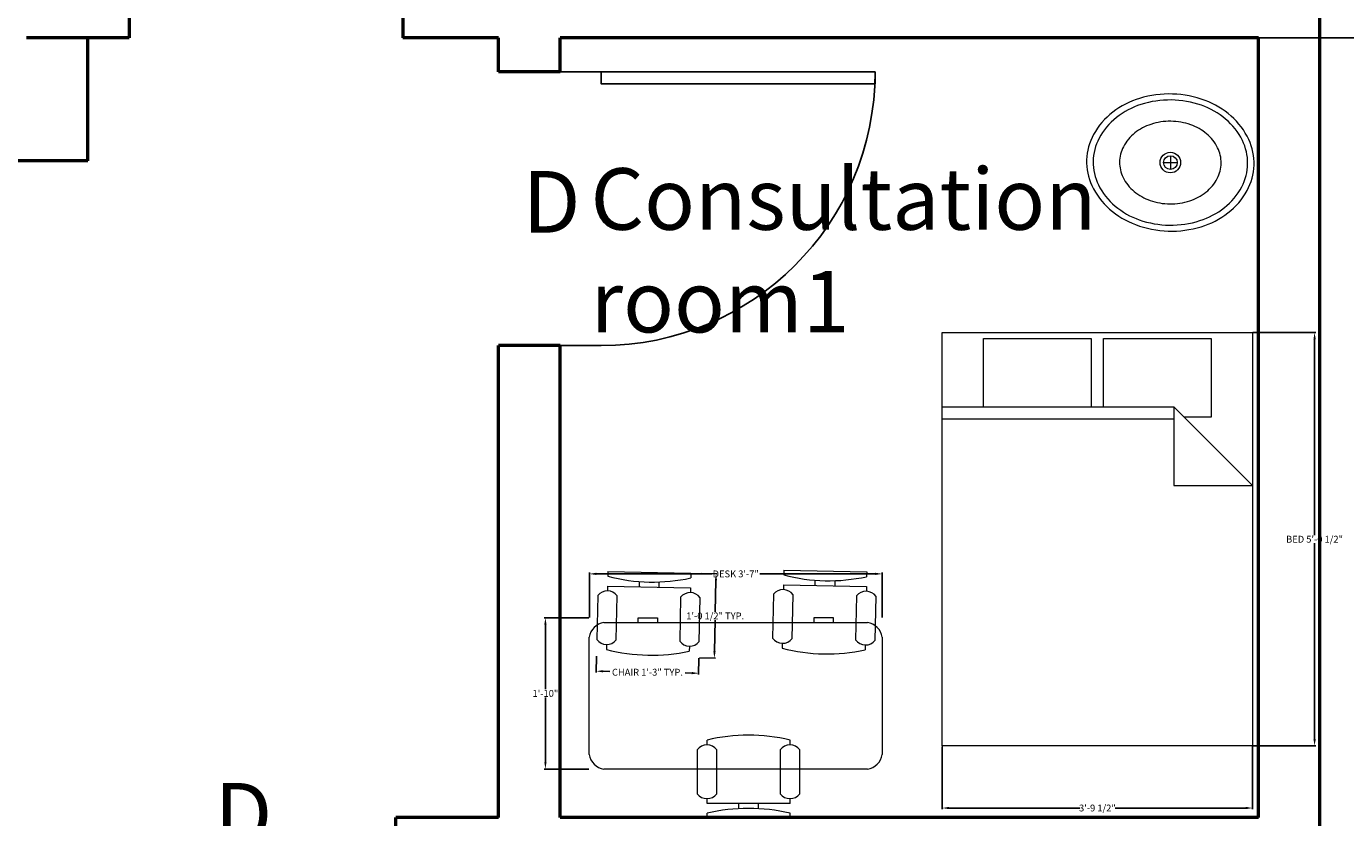
# Model space of a CAD drawing. Units: inches. Extents: x -364 to 705, y -52 to 1250.
# Tile 17 of 34: x 359 to 551, y 417 to 533. Entities that reach past the tile are written whole.
import ezdxf

# ---------------------------------------------------------------- set-up
doc = ezdxf.new("R2010")
doc.units = ezdxf.units.IN
doc.header["$MEASUREMENT"] = 0
for name, color, linetype, lineweight in [('A-ANNO-DIMS', 4, 'Continuous', 18), ('A-ANNO-IDEN', 1, 'Continuous', 18), ('A-AREA-IDEN', 3, 'Continuous', 18), ('A-DOOR', 1, 'Continuous', 25), ('A-FLOR-FIXT', 9, 'Continuous', 18), ('A-FURN', 8, 'Continuous', 18), ('A-WALL', 41, 'Continuous', 50)]:
    doc.layers.add(name, color=color, linetype=linetype, lineweight=lineweight)
doc.styles.get("Standard").update_dxf_attribs({"font": 'arial.ttf'})
doc.dimstyles.get("Standard").update_dxf_attribs({"dimtxt": 1, "dimasz": 1, "dimexe": 0.18, "dimexo": 0.0625, "dimgap": 0.09, "dimtad": 0, "dimtih": 1, "dimtoh": 1, "dimdec": 0, "dimzin": 0, "dimdsep": 46, "dimlunit": 3, "dimtxsty": 'Standard', "dimcen": 0.09, "dimadec": 0, "dimazin": 0, "dimtfac": 1, "dimtdec": 0, "dimtofl": 0, "dimtmove": 0, "dimatfit": 3, "dimfxl": 1, "dimtolj": 1, "dimtzin": 0, "dimarcsym": 0})

# ---------------------------------------------------------------- blocks, each defined once
blk = doc.blocks.new('*U10')
for p, q in [((-40, 0), (-40, 6)), ((0, 0), (0, 6))]:
    blk.add_line(p, q)
blk.add_lwpolyline([(0, 0), (0, -40), (-1.75, -40), (-1.75, 0)], close=True)
blk.add_arc((0, 0), 40, 180, 270)
blk = doc.blocks.new('Chair - Desk')
for p, q in [((-8.5, 0), (-8.5, -1)), ((-8.5, 0), (8.5, 0)), ((8.5, 0), (8.5, -1)), ((-2, -3), (-2, -1.9355)), ((2, -1.9576), (2, -3)), ((-10.5, -5), (-10.5, -14)), ((-8.5, -3), (-8.5, -4)), ((-8.5, -3), (8.5, -3)), ((-6.5, -14), (-6.5, -5)), ((6.5, -5), (6.5, -14)), ((8.5, -3), (8.5, -4)), ((10.5, -14), (10.5, -5)), ((-8.5, -15), (-8.5, -16)), ((8.5, -15), (8.5, -16))]:
    blk.add_line(p, q)
for centre, radius, start, end in [((0, 34.625), 36.625, 256.5803, 283.4197), ((-8.5, -6.5), 2.5, 36.8699, 143.1301), ((8.5, -6.5), 2.5, 36.8699, 143.1301), ((-8.5, -12.5), 2.5, 216.8699, 323.1301), ((0, 19.625), 36.625, 256.5803, 283.4197), ((8.5, -12.5), 2.5, 216.8699, 323.1301)]:
    blk.add_arc(centre, radius, start, end)
blk = doc.blocks.new('Desk - 30 x 60 in.')
for p, q in [((-26.999995, 0), (26.999995, 0)), ((-29.999995, -27), (-29.999995, -3)), ((29.999995, -3), (29.999995, -27)), ((26.999995, -30), (-26.999995, -30)), ((-20.000005, -30), (-20.000005, -31)), ((-20.000005, -31), (-16.000005, -31)), ((-16.000005, -31), (-16.000005, -30)), ((15.999995, -31), (15.999995, -30)), ((19.999995, -31), (15.999995, -31)), ((19.999995, -30), (19.999995, -31))]:
    blk.add_line(p, q)
for centre, start, end in [((-26.499995, -3.5), 98.1301, 171.8699), ((26.499995, -3.5), 8.130102, 81.8699), ((-26.499995, -26.5), 188.1301, 261.8699), ((26.499995, -26.5), 278.1301, 351.8699)]:
    blk.add_arc(centre, 3.535534, start, end)
blk = doc.blocks.new('Bed - Queen')
for p, q in [((0, -80.00003), (0, 0)), ((0, 0), (59.99999, 0)), ((59.99999, 0), (59.99999, -80.00003)), ((7.99999, -1.2), (28.79998, -1.2)), ((7.99999, -14.4), (7.99999, -1.2)), ((28.79998, -1.2), (28.79998, -14.4)), ((31.19999, -1.2), (51.99999, -1.2)), ((31.19999, -14.4), (31.19999, -1.2)), ((51.99999, -1.2), (51.99999, -16.4)), ((0, -14.4), (44.8, -14.4)), ((59.99999, -29.6), (44.8, -14.4)), ((44.8, -14.4), (44.8, -29.6)), ((44.8, -16.8), (0, -16.8)), ((51.99999, -16.4), (46.79936, -16.4)), ((44.8, -29.6), (59.99999, -29.6)), ((59.99999, -80.00003), (0, -80.00003))]:
    blk.add_line(p, q)
blk = doc.blocks.new('Sink - Oval top')
for p, q in [((-1, 0), (1, 0)), ((0, 1), (0, -1))]:
    blk.add_line(p, q)
for points in [[(-12.23, 0.39, 0.117634), (-11.46, -3.36, 0.104469), (-8.88, -6.8, 0.090016), (-5.08, -9.07, 0.08192), (-0.32, -10.02, 0.08192), (4.49, -9.38, 0.090016), (8.42, -7.36, 0.104469), (11.22, -4.09, 0.117634), (12.23, -0.39, 0.117634), (11.46, 3.36, 0.104469), (8.88, 6.8, 0.090016), (5.08, 9.07, 0.08192), (0.32, 10.02, 0.08192), (-4.49, 9.38, 0.090016), (-8.42, 7.36, 0.104469), (-11.22, 4.09, 0.117634)], [(-11.29, 0.16, 0.118622), (-10.52, -3.25, 0.104678), (-8.07, -6.36, 0.089562), (-4.54, -8.37, 0.081185), (-0.13, -9.15, 0.081185), (4.3, -8.49, 0.089562), (7.89, -6.58, 0.104678), (10.42, -3.55, 0.118622), (11.29, -0.16, 0.118622), (10.52, 3.25, 0.104678), (8.07, 6.36, 0.089562), (4.54, 8.37, 0.081185), (0.13, 9.15, 0.081185), (-4.3, 8.49, 0.089562), (-7.89, 6.58, 0.104678), (-10.42, 3.55, 0.118622)], [(-7.42, 0.08, 0.118283), (-6.91, -2.17, 0.104607), (-5.29, -4.21, 0.089718), (-2.97, -5.53, 0.081436), (-0.07, -6.04, 0.081436), (2.84, -5.59, 0.089718), (5.2, -4.33, 0.104607), (6.86, -2.32, 0.118283), (7.42, -0.08, 0.118283), (6.91, 2.17, 0.104607), (5.29, 4.21, 0.089718), (2.97, 5.53, 0.081436), (0.07, 6.04, 0.081436), (-2.84, 5.59, 0.089718), (-5.2, 4.33, 0.104607), (-6.86, 2.32, 0.118283)]]:
    blk.add_lwpolyline(points, format="xyb", close=True)
for radius in [1.5, 1]:
    blk.add_circle((0, 0), radius)
blk = doc.blocks.new('*D38')
at = {"layer": 'A-ANNO-DIMS', "color": 0, "lineweight": -2, "transparency": 16777216}
for p, q in [((441.88, 440.71), (441.83, 438.34)), ((456.85, 440.4), (456.8, 438.04)), ((442.83, 438.5), (443.82, 438.48)), ((455.8, 438.24), (454.82, 438.26))]:
    blk.add_line(p, q, dxfattribs=at)
at = {"layer": 'A-ANNO-DIMS', "color": 0, "transparency": 16777216}
for points in [[(442.83, 438.67), (442.83, 438.34), (441.83, 438.52)], [(455.81, 438.41), (455.8, 438.07), (456.8, 438.22)]]:
    blk.add_solid(points, dxfattribs=at)
at = {"layer": 'Defpoints', "color": 0, "transparency": 16777216}
for p in [(441.88, 440.77), (456.85, 440.47), (456.8, 438.22)]:
    blk.add_point(p, dxfattribs=at)
at = {"layer": 'A-ANNO-DIMS', "color": 0, "transparency": 16777216, "insert": (449.32, 438.37), "char_height": 1, "attachment_point": 5}
blk.add_mtext('\\A1;CHAIR 1\'-3" TYP.', dxfattribs=at)
blk = doc.blocks.new('*D39')
at = {"layer": 'A-ANNO-DIMS', "color": 0, "lineweight": -2, "transparency": 16777216}
for p, q in [((457.16, 452.82), (459.53, 452.77)), ((459.33, 451.78), (459.23, 447.21)), ((459.12, 441.42), (459.21, 445.99)), ((456.91, 440.46), (459.28, 440.42))]:
    blk.add_line(p, q, dxfattribs=at)
at = {"layer": 'A-ANNO-DIMS', "color": 0, "transparency": 16777216}
for points in [[(459.16, 451.78), (459.49, 451.78), (459.35, 452.78)], [(458.95, 441.42), (459.28, 441.42), (459.1, 440.42)]]:
    blk.add_solid(points, dxfattribs=at)
at = {"layer": 'Defpoints', "color": 0, "transparency": 16777216}
for p in [(457.1, 452.82), (459.35, 452.78), (456.85, 440.47)]:
    blk.add_point(p, dxfattribs=at)
at = {"layer": 'A-ANNO-DIMS', "color": 0, "transparency": 16777216, "insert": (459.22, 446.6), "char_height": 1, "attachment_point": 5}
blk.add_mtext('\\A1;1\'-0 1/2" TYP.', dxfattribs=at)
blk = doc.blocks.new('*D48')
at = {"layer": 'A-ANNO-DIMS', "color": 0, "lineweight": -2, "transparency": 16777216}
for p, q in [((440.83, 446.39), (440.83, 452.92)), ((441.83, 452.74), (458.73, 452.74)), ((482.62, 452.74), (465.72, 452.74)), ((483.62, 446.39), (483.62, 452.92))]:
    blk.add_line(p, q, dxfattribs=at)
at = {"layer": 'A-ANNO-DIMS', "color": 0, "transparency": 16777216}
for points in [[(441.83, 452.91), (441.83, 452.58), (440.83, 452.74)], [(482.62, 452.91), (482.62, 452.58), (483.62, 452.74)]]:
    blk.add_solid(points, dxfattribs=at)
at = {"layer": 'Defpoints', "color": 0, "transparency": 16777216}
for p in [(440.83, 452.74), (440.83, 446.33), (483.62, 446.33)]:
    blk.add_point(p, dxfattribs=at)
at = {"layer": 'A-ANNO-DIMS', "color": 0, "transparency": 16777216, "insert": (462.22, 452.74), "char_height": 1, "attachment_point": 5}
blk.add_mtext('\\A1;DESK 3\'-7"', dxfattribs=at)
blk = doc.blocks.new('*D49')
at = {"layer": 'A-ANNO-DIMS', "color": 0, "lineweight": -2, "transparency": 16777216}
for p, q in [((440.77, 446.33), (434.23, 446.33)), ((434.41, 445.33), (434.41, 435.87)), ((434.41, 425.22), (434.41, 434.67)), ((440.77, 424.22), (434.23, 424.22))]:
    blk.add_line(p, q, dxfattribs=at)
at = {"layer": 'A-ANNO-DIMS', "color": 0, "transparency": 16777216}
for points in [[(434.25, 445.33), (434.58, 445.33), (434.41, 446.33)], [(434.25, 425.22), (434.58, 425.22), (434.41, 424.22)]]:
    blk.add_solid(points, dxfattribs=at)
at = {"layer": 'Defpoints', "color": 0, "transparency": 16777216}
for p in [(440.83, 446.33), (434.41, 424.22), (440.83, 424.22)]:
    blk.add_point(p, dxfattribs=at)
at = {"layer": 'A-ANNO-DIMS', "color": 0, "transparency": 16777216, "insert": (434.41, 435.27), "char_height": 1, "attachment_point": 5}
blk.add_mtext('\\A1;1\'-10"', dxfattribs=at)
blk = doc.blocks.new('*D60')
at = {"layer": 'A-ANNO-DIMS', "color": 0, "lineweight": -2, "transparency": 16777216}
for p, q in [((537.79, 488.04), (546.97, 488.04)), ((546.79, 487.04), (546.79, 458.42)), ((546.79, 428.59), (546.79, 457.21)), ((537.79, 427.59), (546.97, 427.59))]:
    blk.add_line(p, q, dxfattribs=at)
at = {"layer": 'A-ANNO-DIMS', "color": 0, "transparency": 16777216}
for points in [[(546.63, 487.04), (546.96, 487.04), (546.79, 488.04)], [(546.63, 428.59), (546.96, 428.59), (546.79, 427.59)]]:
    blk.add_solid(points, dxfattribs=at)
at = {"layer": 'Defpoints', "color": 0, "transparency": 16777216}
for p in [(537.72, 488.04), (546.79, 488.04), (537.72, 427.59)]:
    blk.add_point(p, dxfattribs=at)
at = {"layer": 'A-ANNO-DIMS', "color": 0, "transparency": 16777216, "insert": (546.79, 457.81), "char_height": 1, "attachment_point": 5}
blk.add_mtext('\\A1;BED 5\'-0 1/2"', dxfattribs=at)
blk = doc.blocks.new('*D61')
at = {"layer": 'A-ANNO-DIMS', "color": 0, "lineweight": -2, "transparency": 16777216}
for p, q in [((492.39, 427.53), (492.39, 418.34)), ((537.72, 427.53), (537.72, 418.34)), ((493.39, 418.52), (512.47, 418.52)), ((536.72, 418.52), (517.64, 418.52))]:
    blk.add_line(p, q, dxfattribs=at)
at = {"layer": 'A-ANNO-DIMS', "color": 0, "transparency": 16777216}
for points in [[(493.39, 418.69), (493.39, 418.35), (492.39, 418.52)], [(536.72, 418.69), (536.72, 418.35), (537.72, 418.52)]]:
    blk.add_solid(points, dxfattribs=at)
at = {"layer": 'Defpoints', "color": 0, "transparency": 16777216}
for p in [(492.39, 427.59), (537.72, 427.59), (537.72, 418.52)]:
    blk.add_point(p, dxfattribs=at)
at = {"layer": 'A-ANNO-DIMS', "color": 0, "transparency": 16777216, "insert": (515.06, 418.52), "char_height": 1, "attachment_point": 5}
blk.add_mtext('\\A1;3\'-9 1/2"', dxfattribs=at)
blk = doc.blocks.new('*D80')
at = {"layer": 'A-ANNO-DIMS', "color": 0, "lineweight": -2, "transparency": 16777216}
for p, q in [((538.64, 531.11), (703.01, 531.11)), ((702.83, 530.11), (702.83, 470.22)), ((702.83, 409.11), (702.83, 469.01)), ((538.64, 408.11), (703.01, 408.11))]:
    blk.add_line(p, q, dxfattribs=at)
at = {"layer": 'A-ANNO-DIMS', "color": 0, "transparency": 16777216}
for points in [[(702.66, 530.11), (703, 530.11), (702.83, 531.11)], [(702.66, 409.11), (703, 409.11), (702.83, 408.11)]]:
    blk.add_solid(points, dxfattribs=at)
at = {"layer": 'Defpoints', "color": 0, "transparency": 16777216}
for p in [(538.58, 531.11), (702.83, 531.11), (538.58, 408.11)]:
    blk.add_point(p, dxfattribs=at)
at = {"layer": 'A-ANNO-DIMS', "color": 0, "transparency": 16777216, "insert": (702.83, 469.61), "char_height": 1, "attachment_point": 5}
blk.add_mtext('\\A1;10\'-3"', dxfattribs=at)
blk = doc.blocks.new('*D81')
at = {"layer": 'A-ANNO-DIMS', "color": 0, "lineweight": -2, "transparency": 16777216}
for p, q in [((538.64, 642.11), (703.01, 642.11)), ((702.83, 641.11), (702.83, 587.22)), ((702.83, 532.11), (702.83, 586.01)), ((538.64, 531.11), (703.01, 531.11))]:
    blk.add_line(p, q, dxfattribs=at)
at = {"layer": 'A-ANNO-DIMS', "color": 0, "transparency": 16777216}
for points in [[(702.66, 641.11), (703, 641.11), (702.83, 642.11)], [(702.66, 532.11), (703, 532.11), (702.83, 531.11)]]:
    blk.add_solid(points, dxfattribs=at)
at = {"layer": 'Defpoints', "color": 0, "transparency": 16777216}
for p in [(538.58, 642.11), (702.83, 642.11), (538.58, 531.11)]:
    blk.add_point(p, dxfattribs=at)
at = {"layer": 'A-ANNO-DIMS', "color": 0, "transparency": 16777216, "insert": (702.83, 586.61), "char_height": 1, "attachment_point": 5}
blk.add_mtext('\\A1;9\'-3"', dxfattribs=at)

msp = doc.modelspace()

# ---------------------------------------------------------------- linework, layer by layer
at = {"layer": 'A-WALL'}
for p, q in [((547.58, 11.11), (547.58, 986.11)), ((373.58, 540.11), (373.58, 531.11)), ((413.58, 540.11), (413.58, 531.11)), ((373.58, 531.11), (358.58, 531.11)), ((367.58, 513.11), (367.58, 531.11)), ((427.58, 531.11), (413.58, 531.11)), ((427.58, 526.11), (427.58, 531.11)), ((538.58, 531.11), (436.58, 531.11)), ((436.58, 526.11), (436.58, 531.11)), ((538.58, 417.11), (538.58, 531.11)), ((436.58, 526.11), (427.58, 526.11)), ((367.58, 513.11), (184.58, 513.11)), ((427.58, 417.11), (427.58, 486.11)), ((436.58, 486.11), (427.58, 486.11)), ((436.58, 417.11), (436.58, 486.11)), ((427.58, 417.11), (412.58, 417.11)), ((412.58, 408.11), (412.58, 417.11)), ((538.58, 417.11), (436.58, 417.11))]:
    msp.add_line(p, q, dxfattribs=at)

# ---------------------------------------------------------------- block references
at = {"layer": 'A-DOOR', "rotation": 90}
msp.add_blockref('*U10', (442.58, 526.11), dxfattribs=at)
at = {"layer": 'A-FLOR-FIXT'}
msp.add_blockref('Sink - Oval top', (525.72, 512.86), dxfattribs=at)
at = {"layer": 'A-FURN', "xscale": 0.7556447462569555, "yscale": 0.7556447462569555, "zscale": 0.7556447462569555}
msp.add_blockref('Bed - Queen', (492.39, 488.04), dxfattribs=at)
at = {"layer": 'A-FURN'}
for name, p, xscale, yscale, zscale, rotation in [('Chair - Desk', (449.61, 452.98), 0.713119733074019, 0.713119733074019, 0.713119733074019, 358.8399543093714), ('Chair - Desk', (475.3, 453.17), 0.713119733074019, 0.713119733074019, 0.713119733074019, 358.8399543093714), ('Desk - 30 x 60 in.', (462.22, 424.22), 0.7131197330740192, 0.7131197330740192, 0.7131197330740192, 180), ('Chair - Desk', (464.09, 417.04), 0.7131197330740192, 0.7131197330740192, 0.7131197330740192, 180)]:
    msp.add_blockref(name, p, dxfattribs=dict(at, xscale=xscale, yscale=yscale, zscale=zscale, rotation=rotation))

# ---------------------------------------------------------------- texts
at = {"layer": 'A-ANNO-IDEN', "char_height": 9, "attachment_point": 1}
for insert in [(431.09, 511.62), (386.06, 422.17)]:
    msp.add_mtext_dynamic_manual_height_columns('D', width=16.916, gutter_width=1, heights=[0], dxfattribs=dict(at, insert=insert))
at = {"layer": 'A-AREA-IDEN', "insert": (441, 512.04), "char_height": 9, "attachment_point": 1}
msp.add_mtext_dynamic_manual_height_columns('Consultation room1', width=62.4146, gutter_width=1, heights=[0], dxfattribs=at)

# ---------------------------------------------------------------- dimensions: what is measured, and where the dimension line sits
at = {"layer": 'A-ANNO-DIMS'}
for base, p1, p2, angle, picture, middle in [((702.83, 642.11), (538.58, 531.11), (538.58, 642.11), 90, '*D81', (702.83, 586.61)), ((702.83, 531.11), (538.58, 408.11), (538.58, 531.11), 90, '*D80', (702.83, 469.61)), ((434.41, 424.22), (440.83, 446.33), (440.83, 424.22), 270, '*D49', (434.41, 435.27))]:
    dim = msp.add_linear_dim(base=base, p1=p1, p2=p2, angle=angle, dimstyle='Standard', override={"dimdec": 1, "dimlfac": 1, "dimrnd": 0, "dimzin": 1, "dimdsep": 46, "dimlunit": 4, "dimfrac": 2}, dxfattribs=at)
    dim.commit()
    dim.dimension.update_dxf_attribs({"geometry": picture, "text_midpoint": middle})
for base, p1, p2, angle, text, picture, middle in [((546.7925, 488.0399), (537.7248, 427.5883), (537.7248, 488.0399), 90, 'BED <>', '*D60', (546.7925, 457.8141)), ((440.83, 452.74), (483.62, 446.33), (440.83, 446.33), 180, 'DESK <>', '*D48', (462.22, 452.74)), ((459.35, 452.78), (456.85, 440.47), (457.1, 452.82), 88.84, '<> TYP.', '*D39', (459.22, 446.6)), ((456.8, 438.22), (441.88, 440.77), (456.85, 440.47), 358.84, 'CHAIR <> TYP.', '*D38', (449.32, 438.37))]:
    dim = msp.add_linear_dim(base=base, p1=p1, p2=p2, angle=angle, text=text, dimstyle='Standard', override={"dimdec": 1, "dimlfac": 1, "dimrnd": 0, "dimzin": 1, "dimdsep": 46, "dimlunit": 4, "dimfrac": 2}, dxfattribs=at)
    dim.commit()
    dim.dimension.update_dxf_attribs({"geometry": picture, "text_midpoint": middle})
dim = msp.add_linear_dim(base=(537.72, 418.52), p1=(492.39, 427.59), p2=(537.72, 427.59), dimstyle='Standard', override={"dimdec": 1, "dimlfac": 1, "dimrnd": 0, "dimzin": 1, "dimdsep": 46, "dimlunit": 4, "dimfrac": 2}, dxfattribs=at)
dim.commit()
dim.dimension.update_dxf_attribs({"geometry": '*D61', "text_midpoint": (515.06, 418.52)})

doc.saveas('drawing.dxf')
